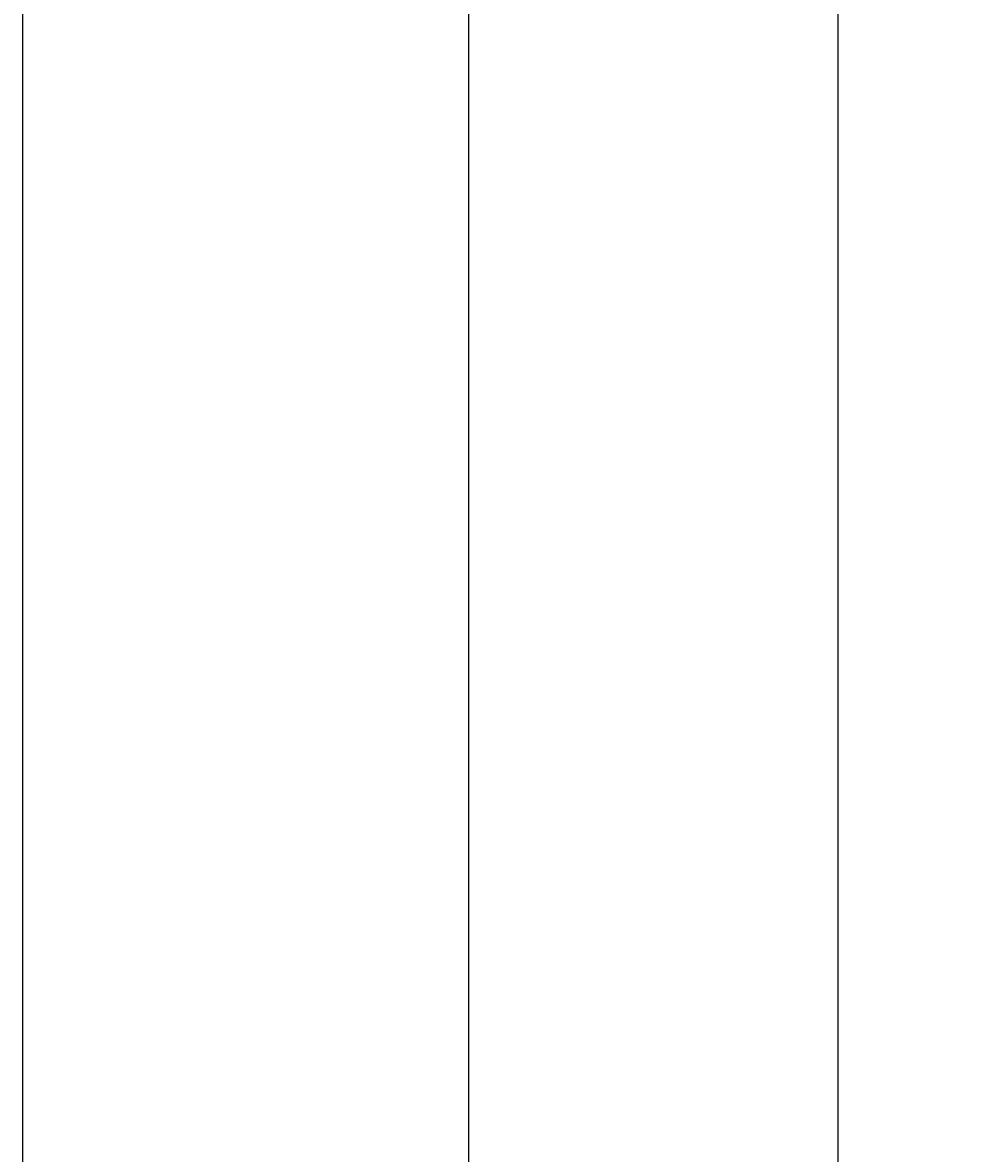
# Model space of a CAD drawing. Units: inches. Extents: x 2812 to 3051, y 1398 to 1659.
# Tile 9 of 65: x 2825 to 2848, y 1501 to 1528. Entities that reach past the tile are written whole.
import ezdxf

# ---------------------------------------------------------------- set-up
doc = ezdxf.new("R2010")
doc.units = ezdxf.units.IN
doc.layers.add('A-ANNO-DIMS', color=2, linetype='Continuous', lineweight=18)
doc.styles.get("Standard").update_dxf_attribs({"font": 'arial.ttf'})
doc.dimstyles.get("Standard").update_dxf_attribs({"dimtxt": 0.18, "dimasz": 0.18, "dimexe": 0.18, "dimexo": 0.0625, "dimgap": 0.09, "dimtad": 0, "dimtih": 1, "dimtoh": 1, "dimdec": 4, "dimzin": 0, "dimdsep": 46, "dimtxsty": 'Standard', "dimcen": 0.09, "dimadec": 0, "dimazin": 0, "dimtfac": 1, "dimtdec": 4, "dimtofl": 0, "dimtmove": 0, "dimatfit": 3, "dimfxl": 1, "dimtolj": 1, "dimtzin": 0, "dimarcsym": 0})

# ---------------------------------------------------------------- blocks, each defined once
blk = doc.blocks.new('*D27')
at = {"layer": 'A-ANNO-DIMS', "color": 0, "lineweight": -2, "transparency": 16777216}
for p, q in [((2824.521, 1594.167), (2824.521, 1397.505)), ((2835.385, 1550.757), (2835.385, 1397.505)), ((2824.701, 1397.685), (2829.498, 1397.685)), ((2835.205, 1397.685), (2830.408, 1397.685))]:
    blk.add_line(p, q, dxfattribs=at)
at = {"layer": 'A-ANNO-DIMS', "color": 0, "transparency": 16777216}
for points in [[(2824.701, 1397.715), (2824.701, 1397.655), (2824.521, 1397.685)], [(2835.205, 1397.715), (2835.205, 1397.655), (2835.385, 1397.685)]]:
    blk.add_solid(points, dxfattribs=at)
at = {"layer": 'Defpoints', "color": 0, "transparency": 16777216}
for p in [(2824.521, 1594.23), (2835.385, 1550.82), (2835.385, 1397.685)]:
    blk.add_point(p, dxfattribs=at)
at = {"layer": 'A-ANNO-DIMS', "color": 0, "transparency": 16777216, "insert": (2829.953, 1397.685), "char_height": 0.18, "attachment_point": 5}
blk.add_mtext('\\A1;10.863', dxfattribs=at)
blk = doc.blocks.new('*D28')
at = {"layer": 'A-ANNO-DIMS', "color": 0, "lineweight": -2, "transparency": 16777216}
for p, q in [((2851.646, 1598.667), (2851.646, 1397.505)), ((2844.385, 1559.757), (2844.385, 1397.505)), ((2844.565, 1397.685), (2847.64, 1397.685)), ((2851.466, 1397.685), (2848.391, 1397.685))]:
    blk.add_line(p, q, dxfattribs=at)
at = {"layer": 'A-ANNO-DIMS', "color": 0, "transparency": 16777216}
for points in [[(2844.565, 1397.715), (2844.565, 1397.655), (2844.385, 1397.685)], [(2851.466, 1397.715), (2851.466, 1397.655), (2851.646, 1397.685)]]:
    blk.add_solid(points, dxfattribs=at)
at = {"layer": 'Defpoints', "color": 0, "transparency": 16777216}
for p in [(2851.646, 1598.73), (2844.385, 1559.82), (2851.646, 1397.685)]:
    blk.add_point(p, dxfattribs=at)
at = {"layer": 'A-ANNO-DIMS', "color": 0, "transparency": 16777216, "insert": (2848.016, 1397.685), "char_height": 0.18, "attachment_point": 5}
blk.add_mtext('\\A1;7.261', dxfattribs=at)

msp = doc.modelspace()

# ---------------------------------------------------------------- dimensions: what is measured, and where the dimension line sits
at = {"layer": 'A-ANNO-DIMS'}
for base, p1, p2, picture, middle in [((2851.6462, 1397.6854), (2844.3849, 1559.82), (2851.6462, 1598.7296), '*D28', (2848.0156, 1397.6854)), ((2835.384907, 1397.685398), (2824.521409, 1594.229631), (2835.384907, 1550.819971), '*D27', (2829.953158, 1397.685398))]:
    dim = msp.add_linear_dim(base=base, p1=p1, p2=p2, dimstyle='Standard', override={"dimdec": 3, "dimlfac": 1, "dimrnd": 0, "dimzin": 0, "dimdsep": 46, "dimlunit": 2}, dxfattribs=at)
    dim.commit()
    dim.dimension.update_dxf_attribs({"geometry": picture, "text_midpoint": middle})

doc.saveas('drawing.dxf')
